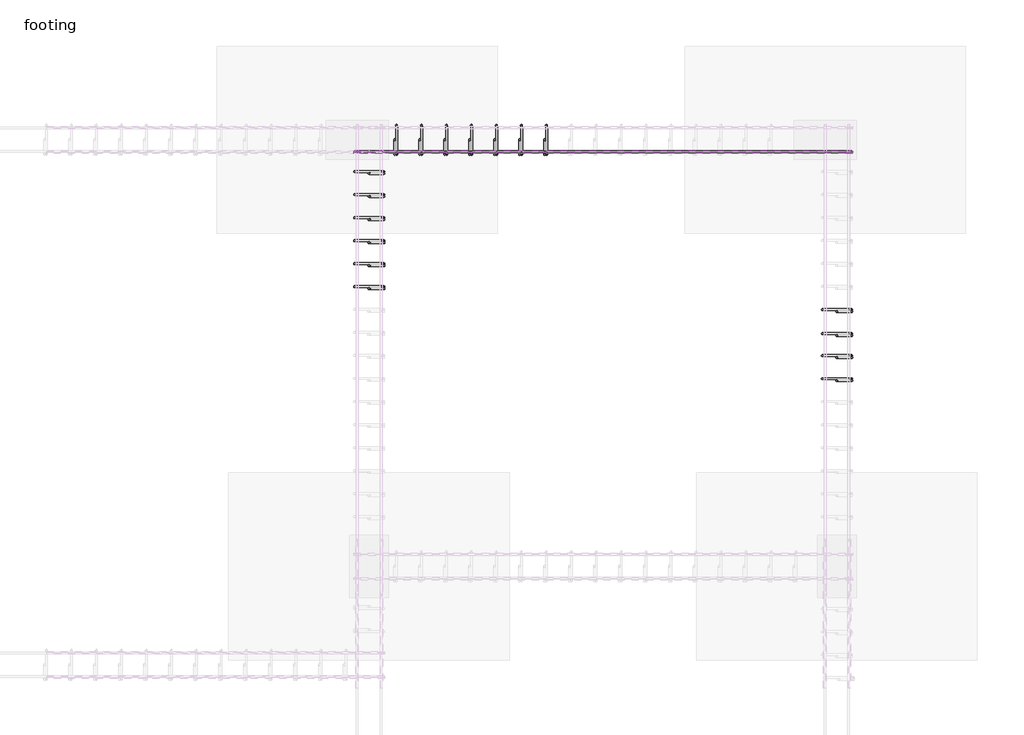
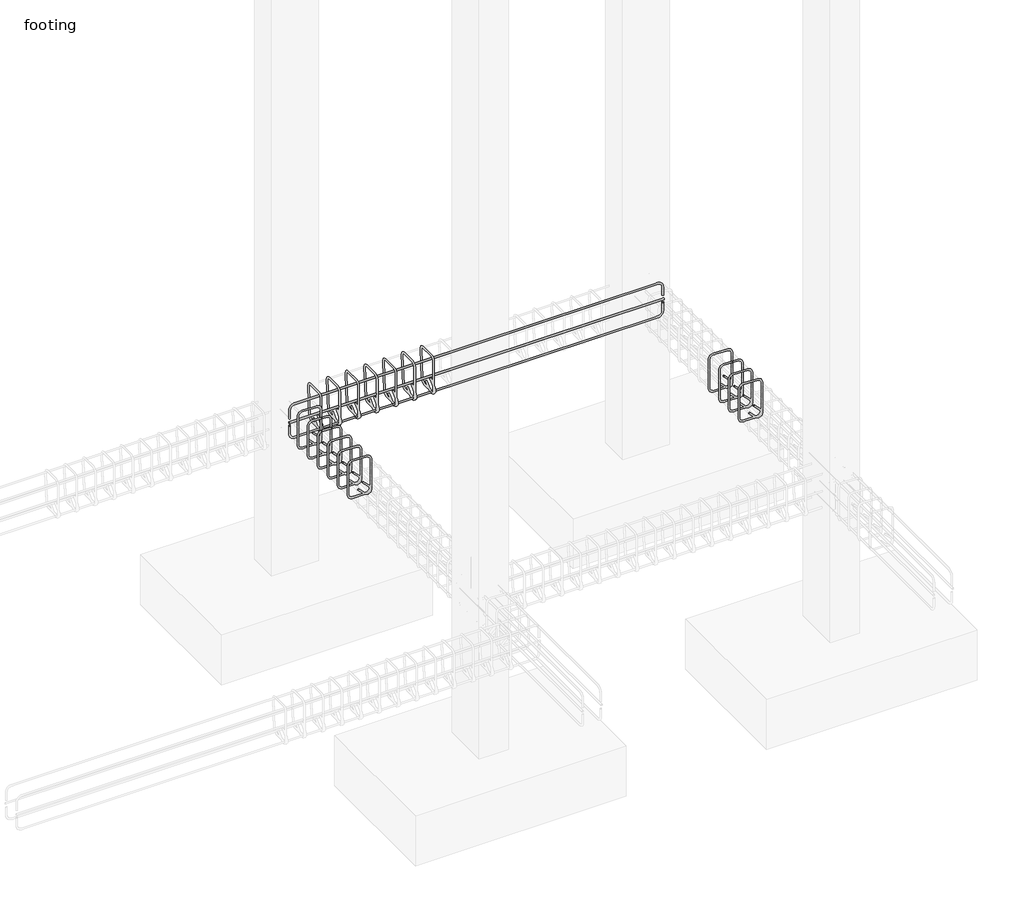
# One storey, part 20 of 21: 20 reinforcing bars.
"""IFC4 building model written with IfcOpenShell, lengths in millimetres."""

from ifc_helpers import new_model, si_unit, point, frame, origin, place, context, project, spatial, polyline, circle_curve, trimmed, segment, composite_curve, element, save
from ifc_brep_helpers import swept_disk

model = new_model("IFC4")

# Units and contexts
model_context = context("Model", 3, world=origin())
ifc_project = project(units=[si_unit("LENGTHUNIT", "METRE", prefix="MILLI")], contexts=[model_context])

# Site, building, storey
site = spatial("IfcSite", under=ifc_project)
building = spatial("IfcBuilding", under=site)
storey = spatial("IfcBuildingStorey", under=building, Name="footing", Elevation=-1524.0)

# Reinforcing bars
placement = place(None, origin())
element("IfcReinforcingBar", 1, at=placement, inside=storey, context=model_context, shape_type="SolidModel", body=[
    swept_disk(composite_curve([segment(polyline([(-7699.7883428, 10994.9387132, -310.8825168), (-7699.7883428, 10940.0737147, -365.7475153)]), True, "CONTINUOUS"), segment(trimmed(circle_curve(frame((-7699.7883428, 10917.6230744, -343.296875), z_axis=(-1.0, 0.0, 0.0), x_axis=(0.0, 22.450640299999577, -22.450640299999975)), 31.75), [point((-7699.7883428, 10940.0737147, -365.7475153))], [point((-7699.7883428, 10885.8730744, -343.296875))], True, "CARTESIAN"), True, "CONTINUOUS"), segment(polyline([(-7699.7883428, 10885.8730744, -343.296875), (-7699.7883428, 10885.8730744, -63.103125)]), True, "CONTINUOUS"), segment(trimmed(circle_curve(frame((-7699.7883428, 10917.6230744, -63.103125), z_axis=(-1.0, 0.0, 0.0), x_axis=(0.0, -31.75, 0.0)), 31.75), [point((-7699.7883428, 10885.8730744, -63.103125))], [point((-7699.7883428, 10917.6230744, -31.353125))], True, "CARTESIAN"), True, "CONTINUOUS"), segment(polyline([(-7699.7883428, 10917.6230744, -31.353125), (-7699.7883428, 11045.4168244, -31.353125)]), True, "CONTINUOUS"), segment(trimmed(circle_curve(frame((-7698.6159328, 11045.4168244, -63.0814712), z_axis=(-0.9993179916193466, 0.0, -0.03692629992126919), x_axis=(-1.1724099999992177, 0.0, 31.728346200000004)), 31.75), [point((-7699.7883428, 11045.4168244, -31.353125))], [point((-7698.6159328, 11077.1668244, -63.0814712))], True, "CARTESIAN"), True, "CONTINUOUS"), segment(polyline([(-7698.6159328, 11077.1668244, -63.0814712), (-7688.2607528, 11077.1668244, -343.3185288)]), True, "CONTINUOUS"), segment(trimmed(circle_curve(frame((-7688.2607528, 11045.4168244, -343.3185288), z_axis=(-0.9993179916193466, 0.0, -0.03692629992126919), x_axis=(0.0, 31.75, 0.0)), 31.75), [point((-7688.2607528, 11077.1668244, -343.3185288))], [point((-7687.0883428, 11045.4168244, -375.046875))], True, "CARTESIAN"), True, "CONTINUOUS"), segment(polyline([(-7687.0883428, 11045.4168244, -375.046875), (-7687.0883428, 10917.6230744, -375.046875)]), True, "CONTINUOUS"), segment(trimmed(circle_curve(frame((-7687.0883428, 10917.6230744, -343.296875), z_axis=(-1.0, 0.0, 0.0), x_axis=(0.0, 0.0, -31.75)), 31.75), [point((-7687.0883428, 10917.6230744, -375.046875))], [point((-7687.0883428, 10895.1724341, -320.8462347))], True, "CARTESIAN"), True, "CONTINUOUS"), segment(polyline([(-7687.0883428, 10895.1724341, -320.8462347), (-7687.0883428, 10950.0374326, -265.9812362)]), True, "CONTINUOUS")], self_intersect=False), 6.35),
])
element("IfcReinforcingBar", 2, at=placement, inside=storey, context=model_context, shape_type="SolidModel", body=[
    swept_disk(composite_curve([segment(polyline([(-4722.5521673, 10904.1526902, -170.2827408), (-4722.5521673, 10904.1526902, -94.0827408)]), True, "CONTINUOUS"), segment(trimmed(circle_curve(frame((-4767.0021673, 10904.1526902, -94.0827408), z_axis=(0.0, -1.0, 0.0), x_axis=(44.44999999999982, 0.0, 0.0)), 44.45), [point((-4722.5521673, 10904.1526902, -94.0827408))], [point((-4767.0021673, 10904.1526902, -49.6327408))], True, "CARTESIAN"), True, "CONTINUOUS"), segment(polyline([(-4767.0021673, 10904.1526902, -49.6327408), (-7917.3959173, 10904.1526902, -49.6327408)]), True, "CONTINUOUS"), segment(trimmed(circle_curve(frame((-7917.3959173, 10904.1526902, -94.0827408), z_axis=(0.0, -1.0, 0.0), x_axis=(0.0, 0.0, 44.449999999999996)), 44.45), [point((-7917.3959173, 10904.1526902, -49.6327408))], [point((-7961.8459173, 10904.1526902, -94.0827408))], True, "CARTESIAN"), True, "CONTINUOUS"), segment(polyline([(-7961.8459173, 10904.1526902, -94.0827408), (-7961.8459173, 10904.1526902, -170.2827408)]), True, "CONTINUOUS")], self_intersect=False), 6.35),
])
element("IfcReinforcingBar", 3, at=placement, inside=storey, context=model_context, shape_type="SolidModel", body=[
    swept_disk(composite_curve([segment(polyline([(-4722.5521673, 10904.1526902, -236.1172592), (-4722.5521673, 10904.1526902, -312.3172592)]), True, "CONTINUOUS"), segment(trimmed(circle_curve(frame((-4767.0021673, 10904.1526902, -312.3172592), z_axis=(0.0, 1.0, 2.1166279873208456e-12), x_axis=(44.44999999999982, 0.0, 0.0)), 44.45), [point((-4722.5521673, 10904.1526902, -312.3172592))], [point((-4767.0021673, 10904.1526902, -356.7672592))], True, "CARTESIAN"), True, "CONTINUOUS"), segment(polyline([(-4767.0021673, 10904.1526902, -356.7672592), (-7917.3959173, 10904.1526902, -356.7672592)]), True, "CONTINUOUS"), segment(trimmed(circle_curve(frame((-7917.3959173, 10904.1526902, -312.3172592), z_axis=(0.0, 1.0, 2.1166279873208456e-12), x_axis=(0.0, 0.0, -44.44999999999999)), 44.45), [point((-7917.3959173, 10904.1526902, -356.7672592))], [point((-7961.8459173, 10904.1526902, -312.3172592))], True, "CARTESIAN"), True, "CONTINUOUS"), segment(polyline([(-7961.8459173, 10904.1526902, -312.3172592), (-7961.8459173, 10904.1526902, -236.1172592)]), True, "CONTINUOUS")], self_intersect=False), 6.35),
])
element("IfcReinforcingBar", 4, at=placement, inside=storey, context=model_context, shape_type="SolidModel", body=[
    swept_disk(composite_curve([segment(polyline([(-4716.2021673, 10898.5730744, -203.2), (-7968.1959173, 10898.5730744, -203.2)]), True, "CONTINUOUS")], self_intersect=False), 6.35),
])
element("IfcReinforcingBar", 5, at=placement, inside=storey, context=model_context, shape_type="SolidModel", body=[
    swept_disk(composite_curve([segment(polyline([(-7537.0883428, 10994.9387132, -310.8825168), (-7537.0883428, 10940.0737147, -365.7475153)]), True, "CONTINUOUS"), segment(trimmed(circle_curve(frame((-7537.0883428, 10917.6230744, -343.296875), z_axis=(-1.0, 0.0, 0.0), x_axis=(0.0, 22.450640299999577, -22.450640299999975)), 31.75), [point((-7537.0883428, 10940.0737147, -365.7475153))], [point((-7537.0883428, 10885.8730744, -343.296875))], True, "CARTESIAN"), True, "CONTINUOUS"), segment(polyline([(-7537.0883428, 10885.8730744, -343.296875), (-7537.0883428, 10885.8730744, -63.103125)]), True, "CONTINUOUS"), segment(trimmed(circle_curve(frame((-7537.0883428, 10917.6230744, -63.103125), z_axis=(-1.0, 0.0, 0.0), x_axis=(0.0, -31.75, 0.0)), 31.75), [point((-7537.0883428, 10885.8730744, -63.103125))], [point((-7537.0883428, 10917.6230744, -31.353125))], True, "CARTESIAN"), True, "CONTINUOUS"), segment(polyline([(-7537.0883428, 10917.6230744, -31.353125), (-7537.0883428, 11045.4168244, -31.353125)]), True, "CONTINUOUS"), segment(trimmed(circle_curve(frame((-7535.9159328, 11045.4168244, -63.0814712), z_axis=(-0.9993179916193466, 0.0, -0.03692629992126919), x_axis=(-1.1724100000001272, 0.0, 31.728346200000004)), 31.75), [point((-7537.0883428, 11045.4168244, -31.353125))], [point((-7535.9159328, 11077.1668244, -63.0814712))], True, "CARTESIAN"), True, "CONTINUOUS"), segment(polyline([(-7535.9159328, 11077.1668244, -63.0814712), (-7525.5607528, 11077.1668244, -343.3185288)]), True, "CONTINUOUS"), segment(trimmed(circle_curve(frame((-7525.5607528, 11045.4168244, -343.3185288), z_axis=(-0.9993179916193466, 0.0, -0.03692629992126919), x_axis=(0.0, 31.75, 0.0)), 31.75), [point((-7525.5607528, 11077.1668244, -343.3185288))], [point((-7524.3883428, 11045.4168244, -375.046875))], True, "CARTESIAN"), True, "CONTINUOUS"), segment(polyline([(-7524.3883428, 11045.4168244, -375.046875), (-7524.3883428, 10917.6230744, -375.046875)]), True, "CONTINUOUS"), segment(trimmed(circle_curve(frame((-7524.3883428, 10917.6230744, -343.296875), z_axis=(-1.0, 0.0, 0.0), x_axis=(0.0, 0.0, -31.75)), 31.75), [point((-7524.3883428, 10917.6230744, -375.046875))], [point((-7524.3883428, 10895.1724341, -320.8462347))], True, "CARTESIAN"), True, "CONTINUOUS"), segment(polyline([(-7524.3883428, 10895.1724341, -320.8462347), (-7524.3883428, 10950.0374326, -265.9812362)]), True, "CONTINUOUS")], self_intersect=False), 6.35),
])
element("IfcReinforcingBar", 6, at=placement, inside=storey, context=model_context, shape_type="SolidModel", body=[
    swept_disk(composite_curve([segment(polyline([(-7374.3883428, 10994.9387132, -310.8825168), (-7374.3883428, 10940.0737147, -365.7475153)]), True, "CONTINUOUS"), segment(trimmed(circle_curve(frame((-7374.3883428, 10917.6230744, -343.296875), z_axis=(-1.0, 0.0, 0.0), x_axis=(0.0, 22.450640299999577, -22.450640299999975)), 31.75), [point((-7374.3883428, 10940.0737147, -365.7475153))], [point((-7374.3883428, 10885.8730744, -343.296875))], True, "CARTESIAN"), True, "CONTINUOUS"), segment(polyline([(-7374.3883428, 10885.8730744, -343.296875), (-7374.3883428, 10885.8730744, -63.103125)]), True, "CONTINUOUS"), segment(trimmed(circle_curve(frame((-7374.3883428, 10917.6230744, -63.103125), z_axis=(-1.0, 0.0, 0.0), x_axis=(0.0, -31.75, 0.0)), 31.75), [point((-7374.3883428, 10885.8730744, -63.103125))], [point((-7374.3883428, 10917.6230744, -31.353125))], True, "CARTESIAN"), True, "CONTINUOUS"), segment(polyline([(-7374.3883428, 10917.6230744, -31.353125), (-7374.3883428, 11045.4168244, -31.353125)]), True, "CONTINUOUS"), segment(trimmed(circle_curve(frame((-7373.2159328, 11045.4168244, -63.0814712), z_axis=(-0.9993179916193466, 0.0, -0.03692629992126919), x_axis=(-1.1724100000001272, 0.0, 31.728346200000004)), 31.75), [point((-7374.3883428, 11045.4168244, -31.353125))], [point((-7373.2159328, 11077.1668244, -63.0814712))], True, "CARTESIAN"), True, "CONTINUOUS"), segment(polyline([(-7373.2159328, 11077.1668244, -63.0814712), (-7362.8607528, 11077.1668244, -343.3185288)]), True, "CONTINUOUS"), segment(trimmed(circle_curve(frame((-7362.8607528, 11045.4168244, -343.3185288), z_axis=(-0.9993179916193466, 0.0, -0.03692629992126919), x_axis=(0.0, 31.75, 0.0)), 31.75), [point((-7362.8607528, 11077.1668244, -343.3185288))], [point((-7361.6883428, 11045.4168244, -375.046875))], True, "CARTESIAN"), True, "CONTINUOUS"), segment(polyline([(-7361.6883428, 11045.4168244, -375.046875), (-7361.6883428, 10917.6230744, -375.046875)]), True, "CONTINUOUS"), segment(trimmed(circle_curve(frame((-7361.6883428, 10917.6230744, -343.296875), z_axis=(-1.0, 0.0, 0.0), x_axis=(0.0, 0.0, -31.75)), 31.75), [point((-7361.6883428, 10917.6230744, -375.046875))], [point((-7361.6883428, 10895.1724341, -320.8462347))], True, "CARTESIAN"), True, "CONTINUOUS"), segment(polyline([(-7361.6883428, 10895.1724341, -320.8462347), (-7361.6883428, 10950.0374326, -265.9812362)]), True, "CONTINUOUS")], self_intersect=False), 6.35),
])
element("IfcReinforcingBar", 7, at=placement, inside=storey, context=model_context, shape_type="SolidModel", body=[
    swept_disk(composite_curve([segment(polyline([(-7211.6883428, 10994.9387132, -310.8825168), (-7211.6883428, 10940.0737147, -365.7475153)]), True, "CONTINUOUS"), segment(trimmed(circle_curve(frame((-7211.6883428, 10917.6230744, -343.296875), z_axis=(-1.0, 0.0, 0.0), x_axis=(0.0, 22.450640299999577, -22.450640299999975)), 31.75), [point((-7211.6883428, 10940.0737147, -365.7475153))], [point((-7211.6883428, 10885.8730744, -343.296875))], True, "CARTESIAN"), True, "CONTINUOUS"), segment(polyline([(-7211.6883428, 10885.8730744, -343.296875), (-7211.6883428, 10885.8730744, -63.103125)]), True, "CONTINUOUS"), segment(trimmed(circle_curve(frame((-7211.6883428, 10917.6230744, -63.103125), z_axis=(-1.0, 0.0, 0.0), x_axis=(0.0, -31.75, 0.0)), 31.75), [point((-7211.6883428, 10885.8730744, -63.103125))], [point((-7211.6883428, 10917.6230744, -31.353125))], True, "CARTESIAN"), True, "CONTINUOUS"), segment(polyline([(-7211.6883428, 10917.6230744, -31.353125), (-7211.6883428, 11045.4168244, -31.353125)]), True, "CONTINUOUS"), segment(trimmed(circle_curve(frame((-7210.5159328, 11045.4168244, -63.0814712), z_axis=(-0.9993179916193466, 0.0, -0.03692629992126919), x_axis=(-1.1724100000001272, 0.0, 31.728346200000004)), 31.75), [point((-7211.6883428, 11045.4168244, -31.353125))], [point((-7210.5159328, 11077.1668244, -63.0814712))], True, "CARTESIAN"), True, "CONTINUOUS"), segment(polyline([(-7210.5159328, 11077.1668244, -63.0814712), (-7200.1607528, 11077.1668244, -343.3185288)]), True, "CONTINUOUS"), segment(trimmed(circle_curve(frame((-7200.1607528, 11045.4168244, -343.3185288), z_axis=(-0.9993179916193466, 0.0, -0.03692629992126919), x_axis=(0.0, 31.75, 0.0)), 31.75), [point((-7200.1607528, 11077.1668244, -343.3185288))], [point((-7198.9883428, 11045.4168244, -375.046875))], True, "CARTESIAN"), True, "CONTINUOUS"), segment(polyline([(-7198.9883428, 11045.4168244, -375.046875), (-7198.9883428, 10917.6230744, -375.046875)]), True, "CONTINUOUS"), segment(trimmed(circle_curve(frame((-7198.9883428, 10917.6230744, -343.296875), z_axis=(-1.0, 0.0, 0.0), x_axis=(0.0, 0.0, -31.75)), 31.75), [point((-7198.9883428, 10917.6230744, -375.046875))], [point((-7198.9883428, 10895.1724341, -320.8462347))], True, "CARTESIAN"), True, "CONTINUOUS"), segment(polyline([(-7198.9883428, 10895.1724341, -320.8462347), (-7198.9883428, 10950.0374326, -265.9812362)]), True, "CONTINUOUS")], self_intersect=False), 6.35),
])
element("IfcReinforcingBar", 8, at=placement, inside=storey, context=model_context, shape_type="SolidModel", body=[
    swept_disk(composite_curve([segment(polyline([(-7048.9883428, 10994.9387132, -310.8825168), (-7048.9883428, 10940.0737147, -365.7475153)]), True, "CONTINUOUS"), segment(trimmed(circle_curve(frame((-7048.9883428, 10917.6230744, -343.296875), z_axis=(-1.0, 0.0, 0.0), x_axis=(0.0, 22.450640299999577, -22.450640299999975)), 31.75), [point((-7048.9883428, 10940.0737147, -365.7475153))], [point((-7048.9883428, 10885.8730744, -343.296875))], True, "CARTESIAN"), True, "CONTINUOUS"), segment(polyline([(-7048.9883428, 10885.8730744, -343.296875), (-7048.9883428, 10885.8730744, -63.103125)]), True, "CONTINUOUS"), segment(trimmed(circle_curve(frame((-7048.9883428, 10917.6230744, -63.103125), z_axis=(-1.0, 0.0, 0.0), x_axis=(0.0, -31.75, 0.0)), 31.75), [point((-7048.9883428, 10885.8730744, -63.103125))], [point((-7048.9883428, 10917.6230744, -31.353125))], True, "CARTESIAN"), True, "CONTINUOUS"), segment(polyline([(-7048.9883428, 10917.6230744, -31.353125), (-7048.9883428, 11045.4168244, -31.353125)]), True, "CONTINUOUS"), segment(trimmed(circle_curve(frame((-7047.8159328, 11045.4168244, -63.0814712), z_axis=(-0.9993179916193466, 0.0, -0.03692629992126919), x_axis=(-1.1724100000001272, 0.0, 31.728346200000004)), 31.75), [point((-7048.9883428, 11045.4168244, -31.353125))], [point((-7047.8159328, 11077.1668244, -63.0814712))], True, "CARTESIAN"), True, "CONTINUOUS"), segment(polyline([(-7047.8159328, 11077.1668244, -63.0814712), (-7037.4607528, 11077.1668244, -343.3185288)]), True, "CONTINUOUS"), segment(trimmed(circle_curve(frame((-7037.4607528, 11045.4168244, -343.3185288), z_axis=(-0.9993179916193466, 0.0, -0.03692629992126919), x_axis=(0.0, 31.75, 0.0)), 31.75), [point((-7037.4607528, 11077.1668244, -343.3185288))], [point((-7036.2883428, 11045.4168244, -375.046875))], True, "CARTESIAN"), True, "CONTINUOUS"), segment(polyline([(-7036.2883428, 11045.4168244, -375.046875), (-7036.2883428, 10917.6230744, -375.046875)]), True, "CONTINUOUS"), segment(trimmed(circle_curve(frame((-7036.2883428, 10917.6230744, -343.296875), z_axis=(-1.0, 0.0, 0.0), x_axis=(0.0, 0.0, -31.75)), 31.75), [point((-7036.2883428, 10917.6230744, -375.046875))], [point((-7036.2883428, 10895.1724341, -320.8462347))], True, "CARTESIAN"), True, "CONTINUOUS"), segment(polyline([(-7036.2883428, 10895.1724341, -320.8462347), (-7036.2883428, 10950.0374326, -265.9812362)]), True, "CONTINUOUS")], self_intersect=False), 6.35),
])
element("IfcReinforcingBar", 9, at=placement, inside=storey, context=model_context, shape_type="SolidModel", body=[
    swept_disk(composite_curve([segment(polyline([(-6886.2883428, 10994.9387132, -310.8825168), (-6886.2883428, 10940.0737147, -365.7475153)]), True, "CONTINUOUS"), segment(trimmed(circle_curve(frame((-6886.2883428, 10917.6230744, -343.296875), z_axis=(-1.0, 0.0, 0.0), x_axis=(0.0, 22.450640299999577, -22.450640299999975)), 31.75), [point((-6886.2883428, 10940.0737147, -365.7475153))], [point((-6886.2883428, 10885.8730744, -343.296875))], True, "CARTESIAN"), True, "CONTINUOUS"), segment(polyline([(-6886.2883428, 10885.8730744, -343.296875), (-6886.2883428, 10885.8730744, -63.103125)]), True, "CONTINUOUS"), segment(trimmed(circle_curve(frame((-6886.2883428, 10917.6230744, -63.103125), z_axis=(-1.0, 0.0, 0.0), x_axis=(0.0, -31.75, 0.0)), 31.75), [point((-6886.2883428, 10885.8730744, -63.103125))], [point((-6886.2883428, 10917.6230744, -31.353125))], True, "CARTESIAN"), True, "CONTINUOUS"), segment(polyline([(-6886.2883428, 10917.6230744, -31.353125), (-6886.2883428, 11045.4168244, -31.353125)]), True, "CONTINUOUS"), segment(trimmed(circle_curve(frame((-6885.1159328, 11045.4168244, -63.0814712), z_axis=(-0.9993179916193466, 0.0, -0.03692629992126919), x_axis=(-1.1724099999992177, 0.0, 31.728346200000004)), 31.75), [point((-6886.2883428, 11045.4168244, -31.353125))], [point((-6885.1159328, 11077.1668244, -63.0814712))], True, "CARTESIAN"), True, "CONTINUOUS"), segment(polyline([(-6885.1159328, 11077.1668244, -63.0814712), (-6874.7607528, 11077.1668244, -343.3185288)]), True, "CONTINUOUS"), segment(trimmed(circle_curve(frame((-6874.7607528, 11045.4168244, -343.3185288), z_axis=(-0.9993179916193466, 0.0, -0.03692629992126919), x_axis=(0.0, 31.75, 0.0)), 31.75), [point((-6874.7607528, 11077.1668244, -343.3185288))], [point((-6873.5883428, 11045.4168244, -375.046875))], True, "CARTESIAN"), True, "CONTINUOUS"), segment(polyline([(-6873.5883428, 11045.4168244, -375.046875), (-6873.5883428, 10917.6230744, -375.046875)]), True, "CONTINUOUS"), segment(trimmed(circle_curve(frame((-6873.5883428, 10917.6230744, -343.296875), z_axis=(-1.0, 0.0, 0.0), x_axis=(0.0, 0.0, -31.75)), 31.75), [point((-6873.5883428, 10917.6230744, -375.046875))], [point((-6873.5883428, 10895.1724341, -320.8462347))], True, "CARTESIAN"), True, "CONTINUOUS"), segment(polyline([(-6873.5883428, 10895.1724341, -320.8462347), (-6873.5883428, 10950.0374326, -265.9812362)]), True, "CONTINUOUS")], self_intersect=False), 6.35),
])
element("IfcReinforcingBar", 10, at=placement, inside=storey, context=model_context, shape_type="SolidModel", body=[
    swept_disk(composite_curve([segment(polyline([(-6723.5883428, 10994.9387132, -310.8825168), (-6723.5883428, 10940.0737147, -365.7475153)]), True, "CONTINUOUS"), segment(trimmed(circle_curve(frame((-6723.5883428, 10917.6230744, -343.296875), z_axis=(-1.0, 0.0, 0.0), x_axis=(0.0, 22.450640299999577, -22.450640299999975)), 31.75), [point((-6723.5883428, 10940.0737147, -365.7475153))], [point((-6723.5883428, 10885.8730744, -343.296875))], True, "CARTESIAN"), True, "CONTINUOUS"), segment(polyline([(-6723.5883428, 10885.8730744, -343.296875), (-6723.5883428, 10885.8730744, -63.103125)]), True, "CONTINUOUS"), segment(trimmed(circle_curve(frame((-6723.5883428, 10917.6230744, -63.103125), z_axis=(-1.0, 0.0, 0.0), x_axis=(0.0, -31.75, 0.0)), 31.75), [point((-6723.5883428, 10885.8730744, -63.103125))], [point((-6723.5883428, 10917.6230744, -31.353125))], True, "CARTESIAN"), True, "CONTINUOUS"), segment(polyline([(-6723.5883428, 10917.6230744, -31.353125), (-6723.5883428, 11045.4168244, -31.353125)]), True, "CONTINUOUS"), segment(trimmed(circle_curve(frame((-6722.4159328, 11045.4168244, -63.0814712), z_axis=(-0.9993179916193466, 0.0, -0.03692629992126919), x_axis=(-1.1724100000001272, 0.0, 31.728346200000004)), 31.75), [point((-6723.5883428, 11045.4168244, -31.353125))], [point((-6722.4159328, 11077.1668244, -63.0814712))], True, "CARTESIAN"), True, "CONTINUOUS"), segment(polyline([(-6722.4159328, 11077.1668244, -63.0814712), (-6712.0607528, 11077.1668244, -343.3185288)]), True, "CONTINUOUS"), segment(trimmed(circle_curve(frame((-6712.0607528, 11045.4168244, -343.3185288), z_axis=(-0.9993179916193466, 0.0, -0.03692629992126919), x_axis=(0.0, 31.75, 0.0)), 31.75), [point((-6712.0607528, 11077.1668244, -343.3185288))], [point((-6710.8883428, 11045.4168244, -375.046875))], True, "CARTESIAN"), True, "CONTINUOUS"), segment(polyline([(-6710.8883428, 11045.4168244, -375.046875), (-6710.8883428, 10917.6230744, -375.046875)]), True, "CONTINUOUS"), segment(trimmed(circle_curve(frame((-6710.8883428, 10917.6230744, -343.296875), z_axis=(-1.0, 0.0, 0.0), x_axis=(0.0, 0.0, -31.75)), 31.75), [point((-6710.8883428, 10917.6230744, -375.046875))], [point((-6710.8883428, 10895.1724341, -320.8462347))], True, "CARTESIAN"), True, "CONTINUOUS"), segment(polyline([(-6710.8883428, 10895.1724341, -320.8462347), (-6710.8883428, 10950.0374326, -265.9812362)]), True, "CONTINUOUS")], self_intersect=False), 6.35),
])
element("IfcReinforcingBar", 11, at=placement, inside=storey, context=model_context, shape_type="SolidModel", body=[
    swept_disk(composite_curve([segment(polyline([(-7834.7165254, 10025.2699494, -265.9812362), (-7779.851527, 10025.2699494, -320.8462347)]), True, "CONTINUOUS"), segment(trimmed(circle_curve(frame((-7802.3021673, 10025.2699494, -343.296875), z_axis=(0.0, 1.0, 0.0), x_axis=(22.450640300000487, 0.0, 22.450640299999975)), 31.75), [point((-7779.851527, 10025.2699494, -320.8462347))], [point((-7802.3021673, 10025.2699494, -375.046875))], True, "CARTESIAN"), True, "CONTINUOUS"), segment(polyline([(-7802.3021673, 10025.2699494, -375.046875), (-7930.0959173, 10025.2699494, -375.046875)]), True, "CONTINUOUS"), segment(trimmed(circle_curve(frame((-7930.0959173, 10025.2699494, -343.296875), z_axis=(0.0, 1.0, 0.0), x_axis=(0.0, 0.0, -31.75)), 31.75), [point((-7930.0959173, 10025.2699494, -375.046875))], [point((-7961.8459173, 10025.2699494, -343.296875))], True, "CARTESIAN"), True, "CONTINUOUS"), segment(polyline([(-7961.8459173, 10025.2699494, -343.296875), (-7961.8459173, 10025.2699494, -63.103125)]), True, "CONTINUOUS"), segment(trimmed(circle_curve(frame((-7930.165658, 10023.1666957, -63.103125), z_axis=(0.06624421176864137, 0.9978034397651431, 0.0), x_axis=(-31.680259300000216, 2.103253700001005, 0.0)), 31.75), [point((-7961.8459173, 10025.2699494, -63.103125))], [point((-7930.165658, 10023.1666957, -31.353125))], True, "CARTESIAN"), True, "CONTINUOUS"), segment(polyline([(-7930.165658, 10023.1666957, -31.353125), (-7802.2324265, 10014.6732031, -31.353125)]), True, "CONTINUOUS"), segment(trimmed(circle_curve(frame((-7802.2324265, 10014.6732031, -63.103125), z_axis=(0.06624421176864137, 0.9978034397651431, 0.0), x_axis=(0.0, 0.0, 31.75)), 31.75), [point((-7802.2324265, 10014.6732031, -31.353125))], [point((-7770.5521673, 10012.5699494, -63.103125))], True, "CARTESIAN"), True, "CONTINUOUS"), segment(polyline([(-7770.5521673, 10012.5699494, -63.103125), (-7770.5521673, 10012.5699494, -343.296875)]), True, "CONTINUOUS"), segment(trimmed(circle_curve(frame((-7802.3021673, 10012.5699494, -343.296875), z_axis=(0.0, 1.0, 0.0), x_axis=(31.75, 0.0, 0.0)), 31.75), [point((-7770.5521673, 10012.5699494, -343.296875))], [point((-7824.7528076, 10012.5699494, -365.7475153))], True, "CARTESIAN"), True, "CONTINUOUS"), segment(polyline([(-7824.7528076, 10012.5699494, -365.7475153), (-7879.617806, 10012.5699494, -310.8825168)]), True, "CONTINUOUS")], self_intersect=False), 6.35),
])
element("IfcReinforcingBar", 12, at=placement, inside=storey, context=model_context, shape_type="SolidModel", body=[
    swept_disk(composite_curve([segment(polyline([(-7834.7165254, 10175.2699494, -265.9812362), (-7779.851527, 10175.2699494, -320.8462347)]), True, "CONTINUOUS"), segment(trimmed(circle_curve(frame((-7802.3021673, 10175.2699494, -343.296875), z_axis=(0.0, 1.0, 0.0), x_axis=(22.450640300000487, 0.0, 22.450640299999975)), 31.75), [point((-7779.851527, 10175.2699494, -320.8462347))], [point((-7802.3021673, 10175.2699494, -375.046875))], True, "CARTESIAN"), True, "CONTINUOUS"), segment(polyline([(-7802.3021673, 10175.2699494, -375.046875), (-7930.0959173, 10175.2699494, -375.046875)]), True, "CONTINUOUS"), segment(trimmed(circle_curve(frame((-7930.0959173, 10175.2699494, -343.296875), z_axis=(0.0, 1.0, 0.0), x_axis=(0.0, 0.0, -31.75)), 31.75), [point((-7930.0959173, 10175.2699494, -375.046875))], [point((-7961.8459173, 10175.2699494, -343.296875))], True, "CARTESIAN"), True, "CONTINUOUS"), segment(polyline([(-7961.8459173, 10175.2699494, -343.296875), (-7961.8459173, 10175.2699494, -63.103125)]), True, "CONTINUOUS"), segment(trimmed(circle_curve(frame((-7930.165658, 10173.1666957, -63.103125), z_axis=(0.06624421176864137, 0.9978034397651431, 0.0), x_axis=(-31.680259300000216, 2.103253700001005, 0.0)), 31.75), [point((-7961.8459173, 10175.2699494, -63.103125))], [point((-7930.165658, 10173.1666957, -31.353125))], True, "CARTESIAN"), True, "CONTINUOUS"), segment(polyline([(-7930.165658, 10173.1666957, -31.353125), (-7802.2324265, 10164.6732031, -31.353125)]), True, "CONTINUOUS"), segment(trimmed(circle_curve(frame((-7802.2324265, 10164.6732031, -63.103125), z_axis=(0.06624421176864137, 0.9978034397651431, 0.0), x_axis=(0.0, 0.0, 31.75)), 31.75), [point((-7802.2324265, 10164.6732031, -31.353125))], [point((-7770.5521673, 10162.5699494, -63.103125))], True, "CARTESIAN"), True, "CONTINUOUS"), segment(polyline([(-7770.5521673, 10162.5699494, -63.103125), (-7770.5521673, 10162.5699494, -343.296875)]), True, "CONTINUOUS"), segment(trimmed(circle_curve(frame((-7802.3021673, 10162.5699494, -343.296875), z_axis=(0.0, 1.0, 0.0), x_axis=(31.75, 0.0, 0.0)), 31.75), [point((-7770.5521673, 10162.5699494, -343.296875))], [point((-7824.7528076, 10162.5699494, -365.7475153))], True, "CARTESIAN"), True, "CONTINUOUS"), segment(polyline([(-7824.7528076, 10162.5699494, -365.7475153), (-7879.617806, 10162.5699494, -310.8825168)]), True, "CONTINUOUS")], self_intersect=False), 6.35),
])
element("IfcReinforcingBar", 13, at=placement, inside=storey, context=model_context, shape_type="SolidModel", body=[
    swept_disk(composite_curve([segment(polyline([(-7834.7165254, 10475.2699494, -265.9812362), (-7779.851527, 10475.2699494, -320.8462347)]), True, "CONTINUOUS"), segment(trimmed(circle_curve(frame((-7802.3021673, 10475.2699494, -343.296875), z_axis=(0.0, 1.0, 0.0), x_axis=(22.450640300000487, 0.0, 22.450640299999975)), 31.75), [point((-7779.851527, 10475.2699494, -320.8462347))], [point((-7802.3021673, 10475.2699494, -375.046875))], True, "CARTESIAN"), True, "CONTINUOUS"), segment(polyline([(-7802.3021673, 10475.2699494, -375.046875), (-7930.0959173, 10475.2699494, -375.046875)]), True, "CONTINUOUS"), segment(trimmed(circle_curve(frame((-7930.0959173, 10475.2699494, -343.296875), z_axis=(0.0, 1.0, 0.0), x_axis=(0.0, 0.0, -31.75)), 31.75), [point((-7930.0959173, 10475.2699494, -375.046875))], [point((-7961.8459173, 10475.2699494, -343.296875))], True, "CARTESIAN"), True, "CONTINUOUS"), segment(polyline([(-7961.8459173, 10475.2699494, -343.296875), (-7961.8459173, 10475.2699494, -63.103125)]), True, "CONTINUOUS"), segment(trimmed(circle_curve(frame((-7930.165658, 10473.1666957, -63.103125), z_axis=(0.06624421176864137, 0.9978034397651431, 0.0), x_axis=(-31.680259300000216, 2.103253700001005, 0.0)), 31.75), [point((-7961.8459173, 10475.2699494, -63.103125))], [point((-7930.165658, 10473.1666957, -31.353125))], True, "CARTESIAN"), True, "CONTINUOUS"), segment(polyline([(-7930.165658, 10473.1666957, -31.353125), (-7802.2324265, 10464.6732031, -31.353125)]), True, "CONTINUOUS"), segment(trimmed(circle_curve(frame((-7802.2324265, 10464.6732031, -63.103125), z_axis=(0.06624421176864137, 0.9978034397651431, 0.0), x_axis=(0.0, 0.0, 31.75)), 31.75), [point((-7802.2324265, 10464.6732031, -31.353125))], [point((-7770.5521673, 10462.5699494, -63.103125))], True, "CARTESIAN"), True, "CONTINUOUS"), segment(polyline([(-7770.5521673, 10462.5699494, -63.103125), (-7770.5521673, 10462.5699494, -343.296875)]), True, "CONTINUOUS"), segment(trimmed(circle_curve(frame((-7802.3021673, 10462.5699494, -343.296875), z_axis=(0.0, 1.0, 0.0), x_axis=(31.75, 0.0, 0.0)), 31.75), [point((-7770.5521673, 10462.5699494, -343.296875))], [point((-7824.7528076, 10462.5699494, -365.7475153))], True, "CARTESIAN"), True, "CONTINUOUS"), segment(polyline([(-7824.7528076, 10462.5699494, -365.7475153), (-7879.617806, 10462.5699494, -310.8825168)]), True, "CONTINUOUS")], self_intersect=False), 6.35),
])
element("IfcReinforcingBar", 14, at=placement, inside=storey, context=model_context, shape_type="SolidModel", body=[
    swept_disk(composite_curve([segment(polyline([(-7834.7165254, 10625.2699494, -265.9812362), (-7779.851527, 10625.2699494, -320.8462347)]), True, "CONTINUOUS"), segment(trimmed(circle_curve(frame((-7802.3021673, 10625.2699494, -343.296875), z_axis=(0.0, 1.0, 0.0), x_axis=(22.450640300000487, 0.0, 22.450640299999975)), 31.75), [point((-7779.851527, 10625.2699494, -320.8462347))], [point((-7802.3021673, 10625.2699494, -375.046875))], True, "CARTESIAN"), True, "CONTINUOUS"), segment(polyline([(-7802.3021673, 10625.2699494, -375.046875), (-7930.0959173, 10625.2699494, -375.046875)]), True, "CONTINUOUS"), segment(trimmed(circle_curve(frame((-7930.0959173, 10625.2699494, -343.296875), z_axis=(0.0, 1.0, 0.0), x_axis=(0.0, 0.0, -31.75)), 31.75), [point((-7930.0959173, 10625.2699494, -375.046875))], [point((-7961.8459173, 10625.2699494, -343.296875))], True, "CARTESIAN"), True, "CONTINUOUS"), segment(polyline([(-7961.8459173, 10625.2699494, -343.296875), (-7961.8459173, 10625.2699494, -63.103125)]), True, "CONTINUOUS"), segment(trimmed(circle_curve(frame((-7930.165658, 10623.1666957, -63.103125), z_axis=(0.06624421176864137, 0.9978034397651431, 0.0), x_axis=(-31.680259300000216, 2.103253700001005, 0.0)), 31.75), [point((-7961.8459173, 10625.2699494, -63.103125))], [point((-7930.165658, 10623.1666957, -31.353125))], True, "CARTESIAN"), True, "CONTINUOUS"), segment(polyline([(-7930.165658, 10623.1666957, -31.353125), (-7802.2324265, 10614.6732031, -31.353125)]), True, "CONTINUOUS"), segment(trimmed(circle_curve(frame((-7802.2324265, 10614.6732031, -63.103125), z_axis=(0.06624421176864137, 0.9978034397651431, 0.0), x_axis=(0.0, 0.0, 31.75)), 31.75), [point((-7802.2324265, 10614.6732031, -31.353125))], [point((-7770.5521673, 10612.5699494, -63.103125))], True, "CARTESIAN"), True, "CONTINUOUS"), segment(polyline([(-7770.5521673, 10612.5699494, -63.103125), (-7770.5521673, 10612.5699494, -343.296875)]), True, "CONTINUOUS"), segment(trimmed(circle_curve(frame((-7802.3021673, 10612.5699494, -343.296875), z_axis=(0.0, 1.0, 0.0), x_axis=(31.75, 0.0, 0.0)), 31.75), [point((-7770.5521673, 10612.5699494, -343.296875))], [point((-7824.7528076, 10612.5699494, -365.7475153))], True, "CARTESIAN"), True, "CONTINUOUS"), segment(polyline([(-7824.7528076, 10612.5699494, -365.7475153), (-7879.617806, 10612.5699494, -310.8825168)]), True, "CONTINUOUS")], self_intersect=False), 6.35),
])
element("IfcReinforcingBar", 15, at=placement, inside=storey, context=model_context, shape_type="SolidModel", body=[
    swept_disk(composite_curve([segment(polyline([(-7834.7165254, 10775.2699494, -265.9812362), (-7779.851527, 10775.2699494, -320.8462347)]), True, "CONTINUOUS"), segment(trimmed(circle_curve(frame((-7802.3021673, 10775.2699494, -343.296875), z_axis=(0.0, 1.0, 0.0), x_axis=(22.450640300000487, 0.0, 22.450640299999975)), 31.75), [point((-7779.851527, 10775.2699494, -320.8462347))], [point((-7802.3021673, 10775.2699494, -375.046875))], True, "CARTESIAN"), True, "CONTINUOUS"), segment(polyline([(-7802.3021673, 10775.2699494, -375.046875), (-7930.0959173, 10775.2699494, -375.046875)]), True, "CONTINUOUS"), segment(trimmed(circle_curve(frame((-7930.0959173, 10775.2699494, -343.296875), z_axis=(0.0, 1.0, 0.0), x_axis=(0.0, 0.0, -31.75)), 31.75), [point((-7930.0959173, 10775.2699494, -375.046875))], [point((-7961.8459173, 10775.2699494, -343.296875))], True, "CARTESIAN"), True, "CONTINUOUS"), segment(polyline([(-7961.8459173, 10775.2699494, -343.296875), (-7961.8459173, 10775.2699494, -63.103125)]), True, "CONTINUOUS"), segment(trimmed(circle_curve(frame((-7930.165658, 10773.1666957, -63.103125), z_axis=(0.06624421176864137, 0.9978034397651431, 0.0), x_axis=(-31.680259300000216, 2.103253700001005, 0.0)), 31.75), [point((-7961.8459173, 10775.2699494, -63.103125))], [point((-7930.165658, 10773.1666957, -31.353125))], True, "CARTESIAN"), True, "CONTINUOUS"), segment(polyline([(-7930.165658, 10773.1666957, -31.353125), (-7802.2324265, 10764.6732031, -31.353125)]), True, "CONTINUOUS"), segment(trimmed(circle_curve(frame((-7802.2324265, 10764.6732031, -63.103125), z_axis=(0.06624421176864137, 0.9978034397651431, 0.0), x_axis=(0.0, 0.0, 31.75)), 31.75), [point((-7802.2324265, 10764.6732031, -31.353125))], [point((-7770.5521673, 10762.5699494, -63.103125))], True, "CARTESIAN"), True, "CONTINUOUS"), segment(polyline([(-7770.5521673, 10762.5699494, -63.103125), (-7770.5521673, 10762.5699494, -343.296875)]), True, "CONTINUOUS"), segment(trimmed(circle_curve(frame((-7802.3021673, 10762.5699494, -343.296875), z_axis=(0.0, 1.0, 0.0), x_axis=(31.75, 0.0, 0.0)), 31.75), [point((-7770.5521673, 10762.5699494, -343.296875))], [point((-7824.7528076, 10762.5699494, -365.7475153))], True, "CARTESIAN"), True, "CONTINUOUS"), segment(polyline([(-7824.7528076, 10762.5699494, -365.7475153), (-7879.617806, 10762.5699494, -310.8825168)]), True, "CONTINUOUS")], self_intersect=False), 6.35),
])
element("IfcReinforcingBar", 16, at=placement, inside=storey, context=model_context, shape_type="SolidModel", body=[
    swept_disk(composite_curve([segment(polyline([(-4786.7165254, 9425.2699494, -265.9812362), (-4731.851527, 9425.2699494, -320.8462347)]), True, "CONTINUOUS"), segment(trimmed(circle_curve(frame((-4754.3021673, 9425.2699494, -343.296875), z_axis=(0.0, 1.0, 0.0), x_axis=(22.450640300000487, 0.0, 22.450640299999975)), 31.75), [point((-4731.851527, 9425.2699494, -320.8462347))], [point((-4754.3021673, 9425.2699494, -375.046875))], True, "CARTESIAN"), True, "CONTINUOUS"), segment(polyline([(-4754.3021673, 9425.2699494, -375.046875), (-4882.0959173, 9425.2699494, -375.046875)]), True, "CONTINUOUS"), segment(trimmed(circle_curve(frame((-4882.0959173, 9425.2699494, -343.296875), z_axis=(0.0, 1.0, 0.0), x_axis=(0.0, 0.0, -31.75)), 31.75), [point((-4882.0959173, 9425.2699494, -375.046875))], [point((-4913.8459173, 9425.2699494, -343.296875))], True, "CARTESIAN"), True, "CONTINUOUS"), segment(polyline([(-4913.8459173, 9425.2699494, -343.296875), (-4913.8459173, 9425.2699494, -63.103125)]), True, "CONTINUOUS"), segment(trimmed(circle_curve(frame((-4882.165658, 9423.1666957, -63.103125), z_axis=(0.06624421176864137, 0.9978034397651431, 0.0), x_axis=(-31.680259300000216, 2.103253700001005, 0.0)), 31.75), [point((-4913.8459173, 9425.2699494, -63.103125))], [point((-4882.165658, 9423.1666957, -31.353125))], True, "CARTESIAN"), True, "CONTINUOUS"), segment(polyline([(-4882.165658, 9423.1666957, -31.353125), (-4754.2324265, 9414.6732031, -31.353125)]), True, "CONTINUOUS"), segment(trimmed(circle_curve(frame((-4754.2324265, 9414.6732031, -63.103125), z_axis=(0.06624421176864137, 0.9978034397651431, 0.0), x_axis=(0.0, 0.0, 31.75)), 31.75), [point((-4754.2324265, 9414.6732031, -31.353125))], [point((-4722.5521673, 9412.5699494, -63.103125))], True, "CARTESIAN"), True, "CONTINUOUS"), segment(polyline([(-4722.5521673, 9412.5699494, -63.103125), (-4722.5521673, 9412.5699494, -343.296875)]), True, "CONTINUOUS"), segment(trimmed(circle_curve(frame((-4754.3021673, 9412.5699494, -343.296875), z_axis=(0.0, 1.0, 0.0), x_axis=(31.75, 0.0, 0.0)), 31.75), [point((-4722.5521673, 9412.5699494, -343.296875))], [point((-4776.7528076, 9412.5699494, -365.7475153))], True, "CARTESIAN"), True, "CONTINUOUS"), segment(polyline([(-4776.7528076, 9412.5699494, -365.7475153), (-4831.617806, 9412.5699494, -310.8825168)]), True, "CONTINUOUS")], self_intersect=False), 6.35),
])
element("IfcReinforcingBar", 17, at=placement, inside=storey, context=model_context, shape_type="SolidModel", body=[
    swept_disk(composite_curve([segment(polyline([(-4786.7165254, 9575.2699494, -265.9812362), (-4731.851527, 9575.2699494, -320.8462347)]), True, "CONTINUOUS"), segment(trimmed(circle_curve(frame((-4754.3021673, 9575.2699494, -343.296875), z_axis=(0.0, 1.0, 0.0), x_axis=(22.450640300000487, 0.0, 22.450640299999975)), 31.75), [point((-4731.851527, 9575.2699494, -320.8462347))], [point((-4754.3021673, 9575.2699494, -375.046875))], True, "CARTESIAN"), True, "CONTINUOUS"), segment(polyline([(-4754.3021673, 9575.2699494, -375.046875), (-4882.0959173, 9575.2699494, -375.046875)]), True, "CONTINUOUS"), segment(trimmed(circle_curve(frame((-4882.0959173, 9575.2699494, -343.296875), z_axis=(0.0, 1.0, 0.0), x_axis=(0.0, 0.0, -31.75)), 31.75), [point((-4882.0959173, 9575.2699494, -375.046875))], [point((-4913.8459173, 9575.2699494, -343.296875))], True, "CARTESIAN"), True, "CONTINUOUS"), segment(polyline([(-4913.8459173, 9575.2699494, -343.296875), (-4913.8459173, 9575.2699494, -63.103125)]), True, "CONTINUOUS"), segment(trimmed(circle_curve(frame((-4882.165658, 9573.1666957, -63.103125), z_axis=(0.06624421176864137, 0.9978034397651431, 0.0), x_axis=(-31.680259300000216, 2.103253700001005, 0.0)), 31.75), [point((-4913.8459173, 9575.2699494, -63.103125))], [point((-4882.165658, 9573.1666957, -31.353125))], True, "CARTESIAN"), True, "CONTINUOUS"), segment(polyline([(-4882.165658, 9573.1666957, -31.353125), (-4754.2324265, 9564.6732031, -31.353125)]), True, "CONTINUOUS"), segment(trimmed(circle_curve(frame((-4754.2324265, 9564.6732031, -63.103125), z_axis=(0.06624421176864137, 0.9978034397651431, 0.0), x_axis=(0.0, 0.0, 31.75)), 31.75), [point((-4754.2324265, 9564.6732031, -31.353125))], [point((-4722.5521673, 9562.5699494, -63.103125))], True, "CARTESIAN"), True, "CONTINUOUS"), segment(polyline([(-4722.5521673, 9562.5699494, -63.103125), (-4722.5521673, 9562.5699494, -343.296875)]), True, "CONTINUOUS"), segment(trimmed(circle_curve(frame((-4754.3021673, 9562.5699494, -343.296875), z_axis=(0.0, 1.0, 0.0), x_axis=(31.75, 0.0, 0.0)), 31.75), [point((-4722.5521673, 9562.5699494, -343.296875))], [point((-4776.7528076, 9562.5699494, -365.7475153))], True, "CARTESIAN"), True, "CONTINUOUS"), segment(polyline([(-4776.7528076, 9562.5699494, -365.7475153), (-4831.617806, 9562.5699494, -310.8825168)]), True, "CONTINUOUS")], self_intersect=False), 6.35),
])
element("IfcReinforcingBar", 18, at=placement, inside=storey, context=model_context, shape_type="SolidModel", body=[
    swept_disk(composite_curve([segment(polyline([(-4786.7165254, 9718.9199494, -265.9812362), (-4731.851527, 9718.9199494, -320.8462347)]), True, "CONTINUOUS"), segment(trimmed(circle_curve(frame((-4754.3021673, 9718.9199494, -343.296875), z_axis=(0.0, 1.0, 0.0), x_axis=(22.450640300000487, 0.0, 22.450640299999975)), 31.75), [point((-4731.851527, 9718.9199494, -320.8462347))], [point((-4754.3021673, 9718.9199494, -375.046875))], True, "CARTESIAN"), True, "CONTINUOUS"), segment(polyline([(-4754.3021673, 9718.9199494, -375.046875), (-4882.0959173, 9718.9199494, -375.046875)]), True, "CONTINUOUS"), segment(trimmed(circle_curve(frame((-4882.0959173, 9718.9199494, -343.296875), z_axis=(0.0, 1.0, 0.0), x_axis=(0.0, 0.0, -31.75)), 31.75), [point((-4882.0959173, 9718.9199494, -375.046875))], [point((-4913.8459173, 9718.9199494, -343.296875))], True, "CARTESIAN"), True, "CONTINUOUS"), segment(polyline([(-4913.8459173, 9718.9199494, -343.296875), (-4913.8459173, 9718.9199494, -63.103125)]), True, "CONTINUOUS"), segment(trimmed(circle_curve(frame((-4882.165658, 9716.8166957, -63.103125), z_axis=(0.06624421176864137, 0.9978034397651431, 0.0), x_axis=(-31.680259300000216, 2.103253700001005, 0.0)), 31.75), [point((-4913.8459173, 9718.9199494, -63.103125))], [point((-4882.165658, 9716.8166957, -31.353125))], True, "CARTESIAN"), True, "CONTINUOUS"), segment(polyline([(-4882.165658, 9716.8166957, -31.353125), (-4754.2324265, 9708.3232031, -31.353125)]), True, "CONTINUOUS"), segment(trimmed(circle_curve(frame((-4754.2324265, 9708.3232031, -63.103125), z_axis=(0.06624421176864137, 0.9978034397651431, 0.0), x_axis=(0.0, 0.0, 31.75)), 31.75), [point((-4754.2324265, 9708.3232031, -31.353125))], [point((-4722.5521673, 9706.2199494, -63.103125))], True, "CARTESIAN"), True, "CONTINUOUS"), segment(polyline([(-4722.5521673, 9706.2199494, -63.103125), (-4722.5521673, 9706.2199494, -343.296875)]), True, "CONTINUOUS"), segment(trimmed(circle_curve(frame((-4754.3021673, 9706.2199494, -343.296875), z_axis=(0.0, 1.0, 0.0), x_axis=(31.75, 0.0, 0.0)), 31.75), [point((-4722.5521673, 9706.2199494, -343.296875))], [point((-4776.7528076, 9706.2199494, -365.7475153))], True, "CARTESIAN"), True, "CONTINUOUS"), segment(polyline([(-4776.7528076, 9706.2199494, -365.7475153), (-4831.617806, 9706.2199494, -310.8825168)]), True, "CONTINUOUS")], self_intersect=False), 6.35),
])
element("IfcReinforcingBar", 19, at=placement, inside=storey, context=model_context, shape_type="SolidModel", body=[
    swept_disk(composite_curve([segment(polyline([(-4786.7165254, 9875.2699494, -265.9812362), (-4731.851527, 9875.2699494, -320.8462347)]), True, "CONTINUOUS"), segment(trimmed(circle_curve(frame((-4754.3021673, 9875.2699494, -343.296875), z_axis=(0.0, 1.0, 0.0), x_axis=(22.450640300000487, 0.0, 22.450640299999975)), 31.75), [point((-4731.851527, 9875.2699494, -320.8462347))], [point((-4754.3021673, 9875.2699494, -375.046875))], True, "CARTESIAN"), True, "CONTINUOUS"), segment(polyline([(-4754.3021673, 9875.2699494, -375.046875), (-4882.0959173, 9875.2699494, -375.046875)]), True, "CONTINUOUS"), segment(trimmed(circle_curve(frame((-4882.0959173, 9875.2699494, -343.296875), z_axis=(0.0, 1.0, 0.0), x_axis=(0.0, 0.0, -31.75)), 31.75), [point((-4882.0959173, 9875.2699494, -375.046875))], [point((-4913.8459173, 9875.2699494, -343.296875))], True, "CARTESIAN"), True, "CONTINUOUS"), segment(polyline([(-4913.8459173, 9875.2699494, -343.296875), (-4913.8459173, 9875.2699494, -63.103125)]), True, "CONTINUOUS"), segment(trimmed(circle_curve(frame((-4882.165658, 9873.1666957, -63.103125), z_axis=(0.06624421176864137, 0.9978034397651431, 0.0), x_axis=(-31.680259300000216, 2.103253700001005, 0.0)), 31.75), [point((-4913.8459173, 9875.2699494, -63.103125))], [point((-4882.165658, 9873.1666957, -31.353125))], True, "CARTESIAN"), True, "CONTINUOUS"), segment(polyline([(-4882.165658, 9873.1666957, -31.353125), (-4754.2324265, 9864.6732031, -31.353125)]), True, "CONTINUOUS"), segment(trimmed(circle_curve(frame((-4754.2324265, 9864.6732031, -63.103125), z_axis=(0.06624421176864137, 0.9978034397651431, 0.0), x_axis=(0.0, 0.0, 31.75)), 31.75), [point((-4754.2324265, 9864.6732031, -31.353125))], [point((-4722.5521673, 9862.5699494, -63.103125))], True, "CARTESIAN"), True, "CONTINUOUS"), segment(polyline([(-4722.5521673, 9862.5699494, -63.103125), (-4722.5521673, 9862.5699494, -343.296875)]), True, "CONTINUOUS"), segment(trimmed(circle_curve(frame((-4754.3021673, 9862.5699494, -343.296875), z_axis=(0.0, 1.0, 0.0), x_axis=(31.75, 0.0, 0.0)), 31.75), [point((-4722.5521673, 9862.5699494, -343.296875))], [point((-4776.7528076, 9862.5699494, -365.7475153))], True, "CARTESIAN"), True, "CONTINUOUS"), segment(polyline([(-4776.7528076, 9862.5699494, -365.7475153), (-4831.617806, 9862.5699494, -310.8825168)]), True, "CONTINUOUS")], self_intersect=False), 6.35),
])
element("IfcReinforcingBar", 20, at=placement, inside=storey, context=model_context, shape_type="SolidModel", body=[
    swept_disk(composite_curve([segment(polyline([(-7834.7165254, 10325.2699494, -265.9812362), (-7779.851527, 10325.2699494, -320.8462347)]), True, "CONTINUOUS"), segment(trimmed(circle_curve(frame((-7802.3021673, 10325.2699494, -343.296875), z_axis=(0.0, 1.0, 0.0), x_axis=(22.450640300000487, 0.0, 22.450640299999975)), 31.75), [point((-7779.851527, 10325.2699494, -320.8462347))], [point((-7802.3021673, 10325.2699494, -375.046875))], True, "CARTESIAN"), True, "CONTINUOUS"), segment(polyline([(-7802.3021673, 10325.2699494, -375.046875), (-7930.0959173, 10325.2699494, -375.046875)]), True, "CONTINUOUS"), segment(trimmed(circle_curve(frame((-7930.0959173, 10325.2699494, -343.296875), z_axis=(0.0, 1.0, 0.0), x_axis=(0.0, 0.0, -31.75)), 31.75), [point((-7930.0959173, 10325.2699494, -375.046875))], [point((-7961.8459173, 10325.2699494, -343.296875))], True, "CARTESIAN"), True, "CONTINUOUS"), segment(polyline([(-7961.8459173, 10325.2699494, -343.296875), (-7961.8459173, 10325.2699494, -63.103125)]), True, "CONTINUOUS"), segment(trimmed(circle_curve(frame((-7930.165658, 10323.1666957, -63.103125), z_axis=(0.06624421176864137, 0.9978034397651431, 0.0), x_axis=(-31.680259300000216, 2.103253700001005, 0.0)), 31.75), [point((-7961.8459173, 10325.2699494, -63.103125))], [point((-7930.165658, 10323.1666957, -31.353125))], True, "CARTESIAN"), True, "CONTINUOUS"), segment(polyline([(-7930.165658, 10323.1666957, -31.353125), (-7802.2324265, 10314.6732031, -31.353125)]), True, "CONTINUOUS"), segment(trimmed(circle_curve(frame((-7802.2324265, 10314.6732031, -63.103125), z_axis=(0.06624421176864137, 0.9978034397651431, 0.0), x_axis=(0.0, 0.0, 31.75)), 31.75), [point((-7802.2324265, 10314.6732031, -31.353125))], [point((-7770.5521673, 10312.5699494, -63.103125))], True, "CARTESIAN"), True, "CONTINUOUS"), segment(polyline([(-7770.5521673, 10312.5699494, -63.103125), (-7770.5521673, 10312.5699494, -343.296875)]), True, "CONTINUOUS"), segment(trimmed(circle_curve(frame((-7802.3021673, 10312.5699494, -343.296875), z_axis=(0.0, 1.0, 0.0), x_axis=(31.75, 0.0, 0.0)), 31.75), [point((-7770.5521673, 10312.5699494, -343.296875))], [point((-7824.7528076, 10312.5699494, -365.7475153))], True, "CARTESIAN"), True, "CONTINUOUS"), segment(polyline([(-7824.7528076, 10312.5699494, -365.7475153), (-7879.617806, 10312.5699494, -310.8825168)]), True, "CONTINUOUS")], self_intersect=False), 6.35),
])

save(model, "model.ifc")

# Revit data of these elements
# Elements 1, 2, 3, 4, 5, 6, 7, 8, 9, 10, 11, 12, 13, 14, 15, 16, 17, 18, 19, 20 (IfcReinforcingBar)
#   Phase Created = New Construction
